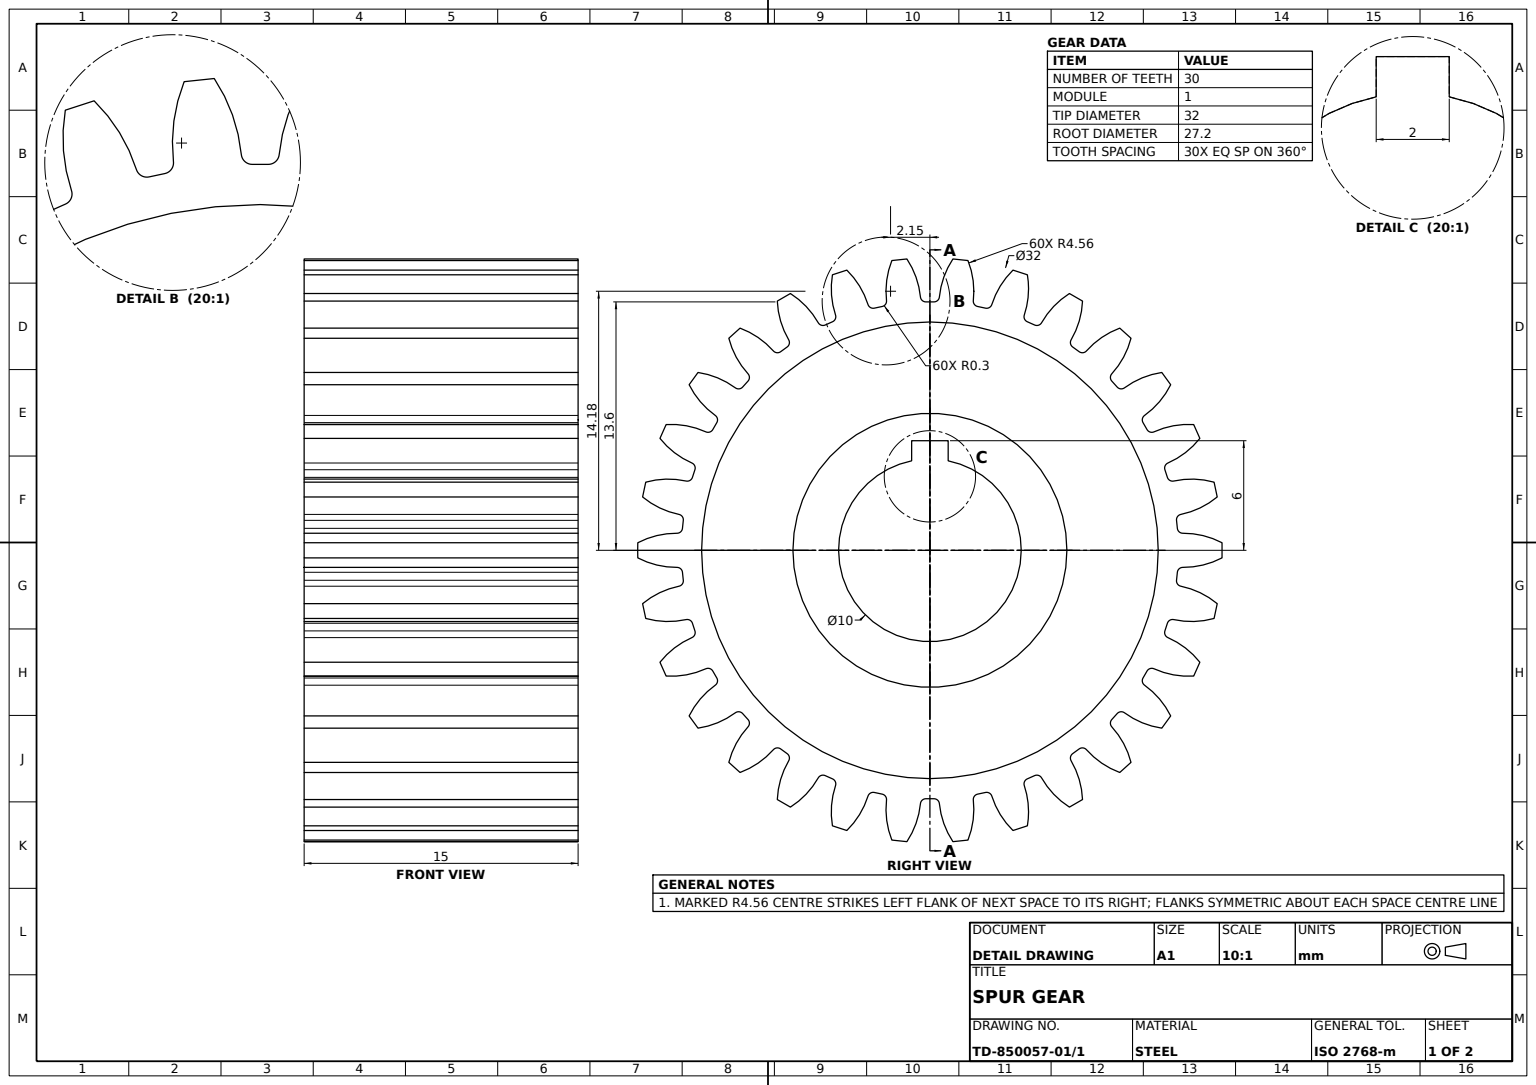
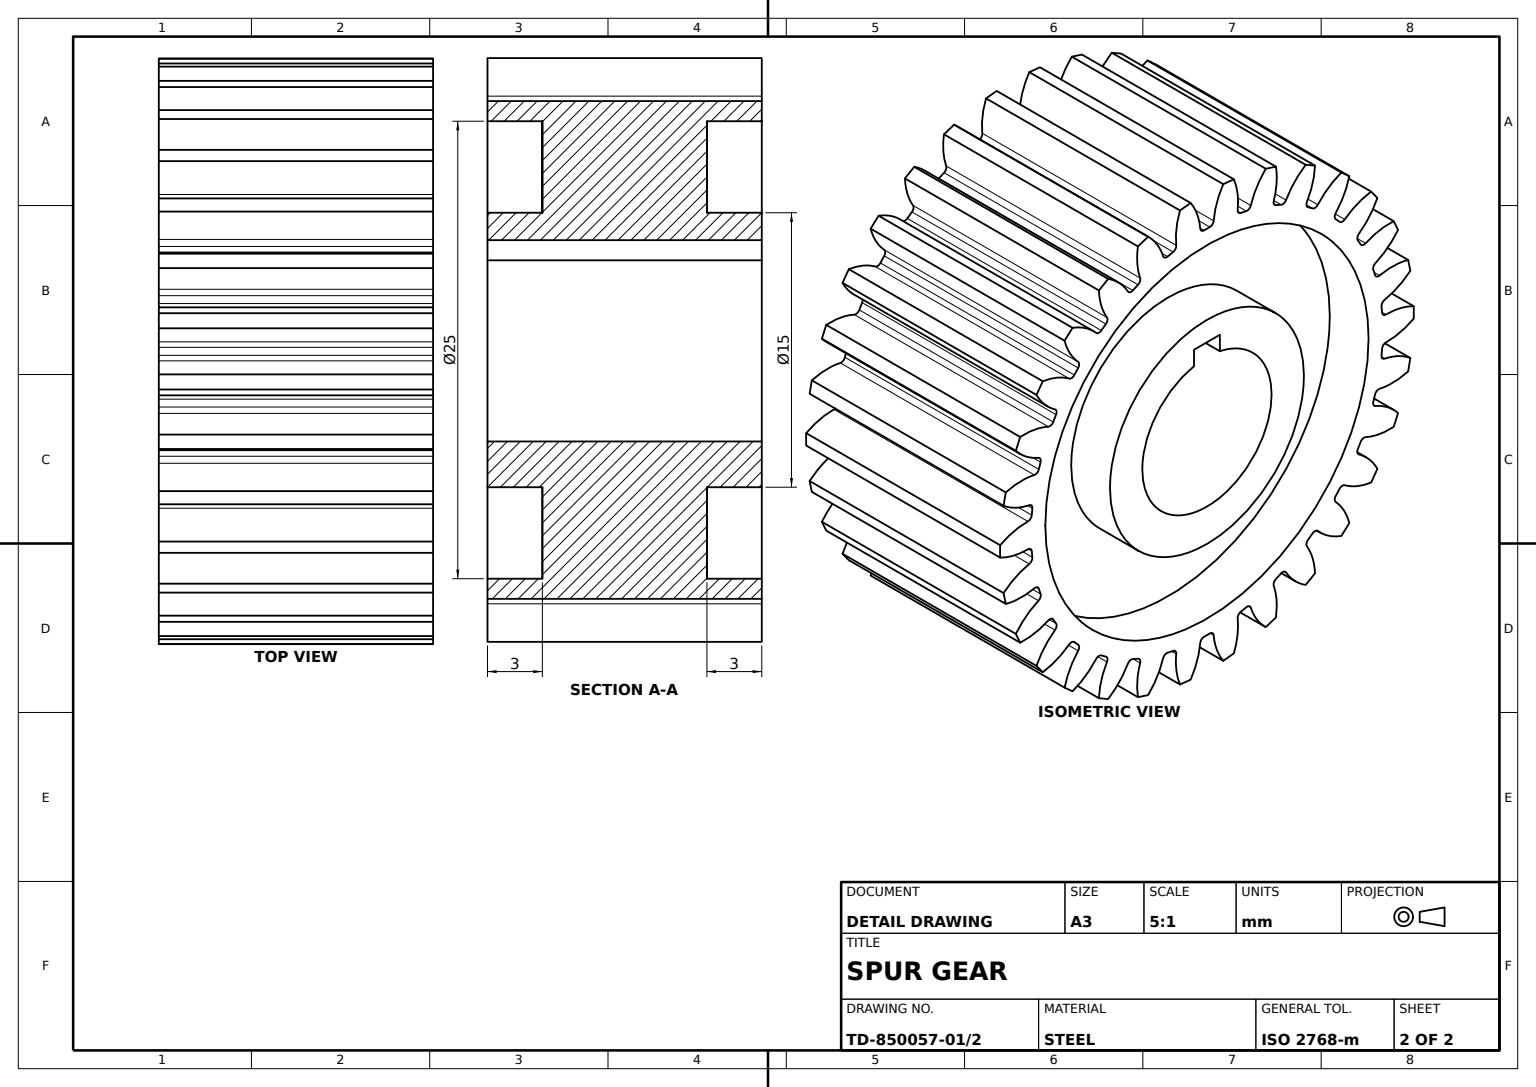
from build123d import *

# Parameters (mm, degrees)
GEAR_BLANK_SKETCH_R       = 16
GEAR_BLANK_32X15_DEPTH    = 7.5
KEYED_BORE_10_DEPTH       = 28.147743921
HUB_RECESS_SKETCH_R       = 12.5
HUB_RECESS_SKETCH_R_2     = 7.5
HUB_RECESS_25_15_X3_DEPTH = 3
TOOTH_SPACE_CUT_DEPTH     = 28.147743921
TOOTH_PATTERN_30X_COUNT   = 30


with BuildPart() as part:
    # Gear Blank Sketch → Gear Blank Ø32x15 (new, symmetric)
    with BuildSketch(Plane(origin=(0, 0, 0), x_dir=(0, 0, -1), z_dir=(1, 0, 0))):
        Circle(GEAR_BLANK_SKETCH_R)
    extrude(amount=GEAR_BLANK_32X15_DEPTH, both=True)

    # Keyed Bore Sketch → Keyed Bore Ø10 (cut, through all)
    with BuildSketch(Plane(origin=(7.5, 0, 0), x_dir=(0, 0, -1), z_dir=(1, 0, 0))):
        with BuildLine():
            Line((-1, 6), (1, 6))
            Line((1, 6), (1, 4.898979486))
            ThreePointArc((1, 4.898979486), (0, -5), (-1, 4.898979486))
            Line((-1, 4.898979486), (-1, 6))
        make_face()
    extrude(amount=-KEYED_BORE_10_DEPTH, mode=Mode.SUBTRACT)

    # Hub Recess Sketch → Hub Recess Ø25-Ø15 x3 (cut)
    with BuildSketch(Plane(origin=(7.5, 0, 0), x_dir=(0, 0, -1), z_dir=(1, 0, 0))):
        Circle(HUB_RECESS_SKETCH_R)
        Circle(HUB_RECESS_SKETCH_R_2, mode=Mode.SUBTRACT)
    hub_recess_25_15_x3 = extrude(amount=-HUB_RECESS_25_15_X3_DEPTH, mode=Mode.SUBTRACT)

    # Hub Recess Mirror: Hub Recess Ø25-Ø15 x3 across plane
    add(hub_recess_25_15_x3.mirror(Plane(origin=(0, 0, 0), x_dir=(0, 0, 1), z_dir=(1, 0, 0))), mode=Mode.SUBTRACT)

    # Tooth Space Sketch → Tooth Space Cut (cut, symmetric)
    with BuildSketch(Plane(origin=(7.5, 0, 0), x_dir=(0, 0, -1), z_dir=(1, 0, 0))):
        with BuildLine():
            Line((-0.219874756, 13.6), (0.219874756, 13.6))
            ThreePointArc((0.219874756, 13.6), (0.421386888, 13.677754953), (0.518441911, 13.870714262))
            ThreePointArc((0.518441911, 13.870714262), (1.009154991, 15.525876188), (2.08, 16.88))
            ThreePointArc((2.08, 16.88), (0, 17.000581665), (-2.08, 16.88))
            ThreePointArc((-2.08, 16.88), (-1.009154991, 15.525876188), (-0.518441911, 13.870714262))
            ThreePointArc((-0.518441911, 13.870714262), (-0.421386888, 13.677754953), (-0.219874756, 13.6))
        make_face()
    tooth_space_cut = extrude(amount=TOOTH_SPACE_CUT_DEPTH, both=True, mode=Mode.SUBTRACT)

    # Tooth Pattern 30x: Tooth Space Cut ×30 about axis
    tooth_pattern_30x_axis = Axis((0, 0, 0), (1, 0, 0))
    for i in range(1, TOOTH_PATTERN_30X_COUNT):
        add(tooth_space_cut.rotate(tooth_pattern_30x_axis, i * 360 / TOOTH_PATTERN_30X_COUNT), mode=Mode.SUBTRACT)


solid = part.part
